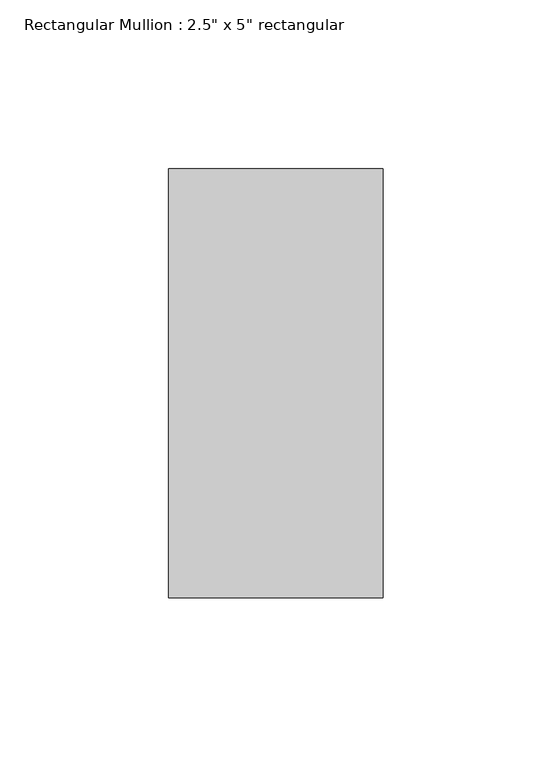
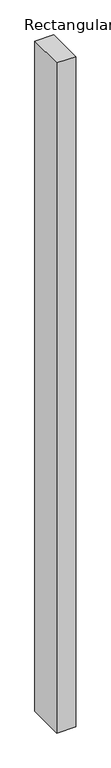
"""IFC4 building model written with IfcOpenShell, lengths in millimetres: member geometry."""

from ifc_helpers import new_model, si_unit, frame, origin, place, context, project, spatial, polyline, outline, extrude, source, transform, mapped, element, save


def member_89bfb2f9(model_context):
    return source(origin(), model_context, "Body", "SweptSolid", [
        extrude(outline(polyline([(31.75, 63.5), (31.75, -63.5), (-31.75, -63.5), (-31.75, 63.5), (31.75, 63.5)])), frame((0.0, 0.0, -2374.9), z_axis=(0.0, 0.0, 1.0), x_axis=(1.0, 0.0, 0.0)), (0.0, 0.0, 1.0), 2374.9),
    ])


if __name__ == "__main__":
    model = new_model("IFC4")
    model_context = context("Model", 3, world=origin())
    ifc_project = project(units=[si_unit("LENGTHUNIT", "METRE", prefix="MILLI")], contexts=[model_context])
    site = spatial("IfcSite", under=ifc_project)
    building = spatial("IfcBuilding", under=site)
    placement = place(None, origin())
    member_shape = member_89bfb2f9(model_context)
    element("IfcMember", 1, ObjectType="Rectangular Mullion : 2.5\" x 5\" rectangular", at=placement, inside=building, context=model_context, shape_type="MappedRepresentation", body=[
        mapped(member_shape, transform((0.0, 0.0, 0.0), x_axis=(1.0, 0.0, 0.0), y_axis=(0.0, 1.0, 0.0), z_axis=(0.0, 0.0, 1.0))),
    ])
    save(model, "model.ifc")

# Revit data of these elements
# Type "Rectangular Mullion : 2.5\" x 5\" rectangular"
#   built-in parameter 1007304 = 0.416667 (stored number, unit not read)
#   built-in parameter 1007301 = 0.104167 (stored number, unit not read)
#   built-in parameter 1007300 = 0.104167 (stored number, unit not read)
# Element 1 (IfcMember, "Rectangular Mullion : 2.5\" x 5\" rectangular")
#   Materials on its faces: "Aluminum"
# Materials
#   "Aluminum": class "Metal", colour RGB 247 247 247, transparency 0, Description = "Aluminum 6061", Cost = 0
